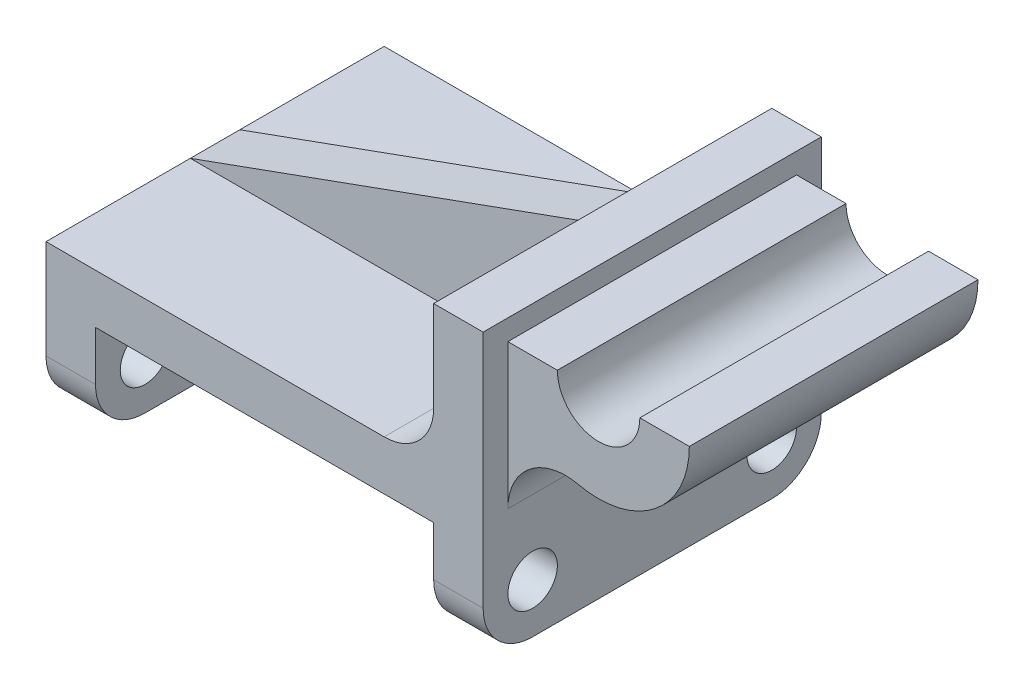
ISO-10303-21;
HEADER;
FILE_DESCRIPTION(('STEP AP214'),'2;1');
FILE_NAME('part.step','',(''),(''),'','','');
FILE_SCHEMA(('AUTOMOTIVE_DESIGN { 1 0 10303 214 1 1 1 1 }'));
ENDSEC;
DATA;
#1=APPLICATION_CONTEXT('core data for automotive mechanical design processes');
#2=APPLICATION_PROTOCOL_DEFINITION('international standard','automotive_design',2000,#1);
#3=PRODUCT_CONTEXT('',#1,'mechanical');
#4=PRODUCT('Part','Part','',(#3));
#5=PRODUCT_RELATED_PRODUCT_CATEGORY('part','',(#4));
#6=PRODUCT_DEFINITION_FORMATION('','',#4);
#7=PRODUCT_DEFINITION_CONTEXT('part definition',#1,'design');
#8=PRODUCT_DEFINITION('design','',#6,#7);
#9=PRODUCT_DEFINITION_SHAPE('','',#8);
#10=(LENGTH_UNIT() NAMED_UNIT(*) SI_UNIT(.MILLI.,.METRE.));
#11=(NAMED_UNIT(*) PLANE_ANGLE_UNIT() SI_UNIT($,.RADIAN.));
#12=(NAMED_UNIT(*) SI_UNIT($,.STERADIAN.) SOLID_ANGLE_UNIT());
#13=UNCERTAINTY_MEASURE_WITH_UNIT(LENGTH_MEASURE(1.E-05),#10,'distance_accuracy_value','');
#14=(GEOMETRIC_REPRESENTATION_CONTEXT(3) GLOBAL_UNCERTAINTY_ASSIGNED_CONTEXT((#13)) GLOBAL_UNIT_ASSIGNED_CONTEXT((#10,
#11,#12)) REPRESENTATION_CONTEXT('',''));
#15=CARTESIAN_POINT('',(0.,0.,0.));
#16=DIRECTION('',(0.,0.,1.));
#17=DIRECTION('',(1.,0.,0.));
#18=AXIS2_PLACEMENT_3D('',#15,#16,#17);
#19=CARTESIAN_POINT('',(0.,36.,0.));
#20=DIRECTION('',(0.,-1.,0.));
#21=DIRECTION('',(0.,0.,-1.));
#22=AXIS2_PLACEMENT_3D('',#19,#20,#21);
#23=PLANE('',#22);
#24=DIRECTION('',(-1.,0.,0.));
#25=VECTOR('',#24,1.);
#26=CARTESIAN_POINT('',(0.,36.,-6.));
#27=LINE('',#26,#25);
#28=CARTESIAN_POINT('',(29.,36.,-6.));
#29=VERTEX_POINT('',#28);
#30=CARTESIAN_POINT('',(-53.,36.,-6.));
#31=VERTEX_POINT('',#30);
#32=EDGE_CURVE('E217',#29,#31,#27,.T.);
#33=ORIENTED_EDGE('',*,*,#32,.F.);
#34=DIRECTION('',(0.,0.,1.));
#35=VECTOR('',#34,1.);
#36=CARTESIAN_POINT('',(29.,36.,0.));
#37=LINE('',#36,#35);
#38=CARTESIAN_POINT('',(29.,36.,-41.));
#39=VERTEX_POINT('',#38);
#40=EDGE_CURVE('E373',#29,#39,#37,.F.);
#41=ORIENTED_EDGE('',*,*,#40,.T.);
#42=DIRECTION('',(-1.,0.,0.));
#43=VECTOR('',#42,1.);
#44=CARTESIAN_POINT('',(-53.,36.,-41.));
#45=LINE('',#44,#43);
#46=CARTESIAN_POINT('',(-53.,36.,-41.));
#47=VERTEX_POINT('',#46);
#48=EDGE_CURVE('E305',#39,#47,#45,.T.);
#49=ORIENTED_EDGE('',*,*,#48,.T.);
#50=DIRECTION('',(0.,0.,1.));
#51=VECTOR('',#50,1.);
#52=CARTESIAN_POINT('',(-53.,36.,41.));
#53=LINE('',#52,#51);
#54=EDGE_CURVE('E306',#47,#31,#53,.T.);
#55=ORIENTED_EDGE('',*,*,#54,.T.);
#56=EDGE_LOOP('',(#33,#41,#49,#55));
#57=FACE_BOUND('',#56,.T.);
#58=ADVANCED_FACE('F43',(#57),#23,.F.);
#59=CARTESIAN_POINT('',(41.,36.,-41.));
#60=DIRECTION('',(-1.,0.,0.));
#61=DIRECTION('',(0.,0.,1.));
#62=AXIS2_PLACEMENT_3D('',#59,#60,#61);
#63=PLANE('',#62);
#64=DIRECTION('',(0.,-1.,0.));
#65=VECTOR('',#64,1.);
#66=CARTESIAN_POINT('',(41.,36.,-41.));
#67=LINE('',#66,#65);
#68=CARTESIAN_POINT('',(41.,70.,-41.));
#69=VERTEX_POINT('',#68);
#70=CARTESIAN_POINT('',(41.,48.,-41.));
#71=VERTEX_POINT('',#70);
#72=EDGE_CURVE('E251',#69,#71,#67,.T.);
#73=ORIENTED_EDGE('',*,*,#72,.T.);
#74=DIRECTION('',(0.,0.,1.));
#75=VECTOR('',#74,1.);
#76=CARTESIAN_POINT('',(41.,48.,-41.));
#77=LINE('',#76,#75);
#78=CARTESIAN_POINT('',(41.,48.,-6.));
#79=VERTEX_POINT('',#78);
#80=EDGE_CURVE('E216',#71,#79,#77,.T.);
#81=ORIENTED_EDGE('',*,*,#80,.T.);
#82=DIRECTION('',(0.,1.,0.));
#83=VECTOR('',#82,1.);
#84=CARTESIAN_POINT('',(41.,36.,-6.));
#85=LINE('',#84,#83);
#86=CARTESIAN_POINT('',(41.,70.,-6.));
#87=VERTEX_POINT('',#86);
#88=EDGE_CURVE('E209',#79,#87,#85,.T.);
#89=ORIENTED_EDGE('',*,*,#88,.T.);
#90=DIRECTION('',(0.,0.,1.));
#91=VECTOR('',#90,1.);
#92=CARTESIAN_POINT('',(41.,70.,-41.));
#93=LINE('',#92,#91);
#94=EDGE_CURVE('E211',#69,#87,#93,.T.);
#95=ORIENTED_EDGE('',*,*,#94,.F.);
#96=EDGE_LOOP('',(#73,#81,#89,#95));
#97=FACE_BOUND('',#96,.T.);
#98=ADVANCED_FACE('F215',(#97),#63,.T.);
#99=CARTESIAN_POINT('',(53.,65.,-35.));
#100=DIRECTION('',(0.,1.,0.));
#101=DIRECTION('',(0.,0.,1.));
#102=AXIS2_PLACEMENT_3D('',#99,#100,#101);
#103=PLANE('',#102);
#104=DIRECTION('',(-1.,0.,0.));
#105=VECTOR('',#104,1.);
#106=CARTESIAN_POINT('',(53.,65.,35.));
#107=LINE('',#106,#105);
#108=CARTESIAN_POINT('',(65.,65.,35.));
#109=VERTEX_POINT('',#108);
#110=CARTESIAN_POINT('',(53.,65.,35.));
#111=VERTEX_POINT('',#110);
#112=EDGE_CURVE('E429',#109,#111,#107,.T.);
#113=ORIENTED_EDGE('',*,*,#112,.F.);
#114=DIRECTION('',(0.,0.,1.));
#115=VECTOR('',#114,1.);
#116=CARTESIAN_POINT('',(65.,65.,-47.));
#117=LINE('',#116,#115);
#118=CARTESIAN_POINT('',(65.,65.,-35.));
#119=VERTEX_POINT('',#118);
#120=EDGE_CURVE('E401',#119,#109,#117,.T.);
#121=ORIENTED_EDGE('',*,*,#120,.F.);
#122=DIRECTION('',(-1.,0.,0.));
#123=VECTOR('',#122,1.);
#124=CARTESIAN_POINT('',(53.,65.,-35.));
#125=LINE('',#124,#123);
#126=CARTESIAN_POINT('',(53.,65.,-35.));
#127=VERTEX_POINT('',#126);
#128=EDGE_CURVE('E417',#119,#127,#125,.T.);
#129=ORIENTED_EDGE('',*,*,#128,.T.);
#130=DIRECTION('',(0.,0.,1.));
#131=VECTOR('',#130,1.);
#132=CARTESIAN_POINT('',(53.,65.,-35.));
#133=LINE('',#132,#131);
#134=EDGE_CURVE('E435',#127,#111,#133,.T.);
#135=ORIENTED_EDGE('',*,*,#134,.T.);
#136=EDGE_LOOP('',(#113,#121,#129,#135));
#137=FACE_BOUND('',#136,.T.);
#138=ADVANCED_FACE('F518',(#137),#103,.T.);
#139=CARTESIAN_POINT('',(53.,36.,41.));
#140=DIRECTION('',(-1.,0.,0.));
#141=DIRECTION('',(0.,0.,1.));
#142=AXIS2_PLACEMENT_3D('',#139,#140,#141);
#143=PLANE('',#142);
#144=DIRECTION('',(0.,0.,1.));
#145=VECTOR('',#144,1.);
#146=CARTESIAN_POINT('',(53.,29.9001424504315,-35.));
#147=LINE('',#146,#145);
#148=CARTESIAN_POINT('',(53.,29.9001424504315,-35.));
#149=VERTEX_POINT('',#148);
#150=CARTESIAN_POINT('',(53.,29.9001424504315,35.));
#151=VERTEX_POINT('',#150);
#152=EDGE_CURVE('E418',#149,#151,#147,.T.);
#153=ORIENTED_EDGE('',*,*,#152,.T.);
#154=DIRECTION('',(0.,-1.,0.));
#155=VECTOR('',#154,1.);
#156=CARTESIAN_POINT('',(53.,29.9001424504315,35.));
#157=LINE('',#156,#155);
#158=EDGE_CURVE('E403',#111,#151,#157,.T.);
#159=ORIENTED_EDGE('',*,*,#158,.F.);
#160=ORIENTED_EDGE('',*,*,#134,.F.);
#161=DIRECTION('',(0.,-1.,0.));
#162=VECTOR('',#161,1.);
#163=CARTESIAN_POINT('',(53.,29.9001424504315,-35.));
#164=LINE('',#163,#162);
#165=EDGE_CURVE('E407',#127,#149,#164,.T.);
#166=ORIENTED_EDGE('',*,*,#165,.T.);
#167=EDGE_LOOP('',(#153,#159,#160,#166));
#168=FACE_BOUND('',#167,.T.);
#169=CARTESIAN_POINT('',(53.,12.,29.));
#170=DIRECTION('',(-1.,0.,0.));
#171=DIRECTION('',(0.,0.,1.));
#172=AXIS2_PLACEMENT_3D('',#169,#170,#171);
#173=CIRCLE('',#172,6.00000000000001);
#174=CARTESIAN_POINT('',(53.,12.,35.));
#175=VERTEX_POINT('',#174);
#176=EDGE_CURVE('E258',#175,#175,#173,.T.);
#177=ORIENTED_EDGE('',*,*,#176,.T.);
#178=EDGE_LOOP('',(#177));
#179=FACE_BOUND('',#178,.T.);
#180=DIRECTION('',(0.,0.,-1.));
#181=VECTOR('',#180,1.);
#182=CARTESIAN_POINT('',(53.,0.,41.));
#183=LINE('',#182,#181);
#184=CARTESIAN_POINT('',(53.,0.,29.));
#185=VERTEX_POINT('',#184);
#186=CARTESIAN_POINT('',(53.,0.,-29.));
#187=VERTEX_POINT('',#186);
#188=EDGE_CURVE('E298',#185,#187,#183,.T.);
#189=ORIENTED_EDGE('',*,*,#188,.T.);
#190=CARTESIAN_POINT('',(53.,12.,-29.));
#191=DIRECTION('',(-1.,0.,0.));
#192=DIRECTION('',(0.,0.,1.));
#193=AXIS2_PLACEMENT_3D('',#190,#191,#192);
#194=CIRCLE('',#193,12.);
#195=CARTESIAN_POINT('',(53.,12.,-41.));
#196=VERTEX_POINT('',#195);
#197=EDGE_CURVE('E345',#187,#196,#194,.F.);
#198=ORIENTED_EDGE('',*,*,#197,.T.);
#199=DIRECTION('',(0.,-1.,0.));
#200=VECTOR('',#199,1.);
#201=CARTESIAN_POINT('',(53.,36.,-41.));
#202=LINE('',#201,#200);
#203=CARTESIAN_POINT('',(53.,70.,-41.));
#204=VERTEX_POINT('',#203);
#205=EDGE_CURVE('E322',#204,#196,#202,.T.);
#206=ORIENTED_EDGE('',*,*,#205,.F.);
#207=DIRECTION('',(0.,0.,1.));
#208=VECTOR('',#207,1.);
#209=CARTESIAN_POINT('',(53.,70.,-41.));
#210=LINE('',#209,#208);
#211=CARTESIAN_POINT('',(53.,70.,41.));
#212=VERTEX_POINT('',#211);
#213=EDGE_CURVE('E255',#204,#212,#210,.T.);
#214=ORIENTED_EDGE('',*,*,#213,.T.);
#215=DIRECTION('',(0.,-1.,0.));
#216=VECTOR('',#215,1.);
#217=CARTESIAN_POINT('',(53.,36.,41.));
#218=LINE('',#217,#216);
#219=CARTESIAN_POINT('',(53.,12.,41.));
#220=VERTEX_POINT('',#219);
#221=EDGE_CURVE('E311',#212,#220,#218,.T.);
#222=ORIENTED_EDGE('',*,*,#221,.T.);
#223=CARTESIAN_POINT('',(53.,12.,29.));
#224=DIRECTION('',(-1.,0.,0.));
#225=DIRECTION('',(0.,0.,1.));
#226=AXIS2_PLACEMENT_3D('',#223,#224,#225);
#227=CIRCLE('',#226,12.);
#228=EDGE_CURVE('E338',#220,#185,#227,.F.);
#229=ORIENTED_EDGE('',*,*,#228,.T.);
#230=EDGE_LOOP('',(#189,#198,#206,#214,#222,#229));
#231=FACE_BOUND('',#230,.T.);
#232=CARTESIAN_POINT('',(53.,12.,-29.));
#233=DIRECTION('',(-1.,0.,0.));
#234=DIRECTION('',(0.,0.,1.));
#235=AXIS2_PLACEMENT_3D('',#232,#233,#234);
#236=CIRCLE('',#235,6.);
#237=CARTESIAN_POINT('',(53.,12.,-23.));
#238=VERTEX_POINT('',#237);
#239=EDGE_CURVE('E247',#238,#238,#236,.T.);
#240=ORIENTED_EDGE('',*,*,#239,.T.);
#241=EDGE_LOOP('',(#240));
#242=FACE_BOUND('',#241,.T.);
#243=ADVANCED_FACE('F488',(#168,#179,#231,#242),#143,.F.);
#244=DIRECTION('',(1.,0.,0.));
#245=VECTOR('',#244,1.);
#246=CARTESIAN_POINT('',(-53.,36.,41.));
#247=LINE('',#246,#245);
#248=CARTESIAN_POINT('',(-53.,36.,41.));
#249=VERTEX_POINT('',#248);
#250=CARTESIAN_POINT('',(29.,36.,41.));
#251=VERTEX_POINT('',#250);
#252=EDGE_CURVE('E307',#249,#251,#247,.T.);
#253=ORIENTED_EDGE('',*,*,#252,.T.);
#254=DIRECTION('',(0.,0.,1.));
#255=VECTOR('',#254,1.);
#256=CARTESIAN_POINT('',(29.,36.,0.));
#257=LINE('',#256,#255);
#258=CARTESIAN_POINT('',(29.,36.,6.));
#259=VERTEX_POINT('',#258);
#260=EDGE_CURVE('E64',#251,#259,#257,.F.);
#261=ORIENTED_EDGE('',*,*,#260,.T.);
#262=DIRECTION('',(-1.,0.,0.));
#263=VECTOR('',#262,1.);
#264=CARTESIAN_POINT('',(0.,36.,6.));
#265=LINE('',#264,#263);
#266=CARTESIAN_POINT('',(-53.,36.,6.));
#267=VERTEX_POINT('',#266);
#268=EDGE_CURVE('E391',#259,#267,#265,.T.);
#269=ORIENTED_EDGE('',*,*,#268,.T.);
#270=EDGE_CURVE('E302',#267,#249,#53,.T.);
#271=ORIENTED_EDGE('',*,*,#270,.T.);
#272=EDGE_LOOP('',(#253,#261,#269,#271));
#273=FACE_BOUND('',#272,.T.);
#274=ADVANCED_FACE('F451',(#273),#23,.F.);
#275=CARTESIAN_POINT('',(0.,0.,0.));
#276=DIRECTION('',(0.,-1.,0.));
#277=DIRECTION('',(0.,0.,-1.));
#278=AXIS2_PLACEMENT_3D('',#275,#276,#277);
#279=PLANE('',#278);
#280=DIRECTION('',(1.,0.,0.));
#281=VECTOR('',#280,1.);
#282=CARTESIAN_POINT('',(-53.,0.,29.));
#283=LINE('',#282,#281);
#284=CARTESIAN_POINT('',(-41.,0.,29.));
#285=VERTEX_POINT('',#284);
#286=CARTESIAN_POINT('',(-53.,0.,29.));
#287=VERTEX_POINT('',#286);
#288=EDGE_CURVE('E351',#285,#287,#283,.F.);
#289=ORIENTED_EDGE('',*,*,#288,.T.);
#290=DIRECTION('',(0.,0.,1.));
#291=VECTOR('',#290,1.);
#292=CARTESIAN_POINT('',(-53.,0.,41.));
#293=LINE('',#292,#291);
#294=CARTESIAN_POINT('',(-53.,0.,-29.));
#295=VERTEX_POINT('',#294);
#296=EDGE_CURVE('E304',#295,#287,#293,.T.);
#297=ORIENTED_EDGE('',*,*,#296,.F.);
#298=DIRECTION('',(-1.,0.,0.));
#299=VECTOR('',#298,1.);
#300=CARTESIAN_POINT('',(-41.,0.,-29.));
#301=LINE('',#300,#299);
#302=CARTESIAN_POINT('',(-41.,0.,-29.));
#303=VERTEX_POINT('',#302);
#304=EDGE_CURVE('E357',#295,#303,#301,.F.);
#305=ORIENTED_EDGE('',*,*,#304,.T.);
#306=DIRECTION('',(0.,0.,1.));
#307=VECTOR('',#306,1.);
#308=CARTESIAN_POINT('',(-41.,0.,-41.));
#309=LINE('',#308,#307);
#310=EDGE_CURVE('E287',#303,#285,#309,.T.);
#311=ORIENTED_EDGE('',*,*,#310,.T.);
#312=EDGE_LOOP('',(#289,#297,#305,#311));
#313=FACE_BOUND('',#312,.T.);
#314=ADVANCED_FACE('F505',(#313),#279,.T.);
#315=CARTESIAN_POINT('',(-53.,36.,-41.));
#316=DIRECTION('',(0.,0.,1.));
#317=DIRECTION('',(1.,0.,0.));
#318=AXIS2_PLACEMENT_3D('',#315,#316,#317);
#319=PLANE('',#318);
#320=ORIENTED_EDGE('',*,*,#205,.T.);
#321=DIRECTION('',(-1.,0.,0.));
#322=VECTOR('',#321,1.);
#323=CARTESIAN_POINT('',(41.,12.,-41.));
#324=LINE('',#323,#322);
#325=CARTESIAN_POINT('',(41.,12.,-41.));
#326=VERTEX_POINT('',#325);
#327=EDGE_CURVE('E326',#196,#326,#324,.T.);
#328=ORIENTED_EDGE('',*,*,#327,.T.);
#329=DIRECTION('',(0.,1.,0.));
#330=VECTOR('',#329,1.);
#331=CARTESIAN_POINT('',(41.,0.,-41.));
#332=LINE('',#331,#330);
#333=CARTESIAN_POINT('',(41.,24.,-41.));
#334=VERTEX_POINT('',#333);
#335=EDGE_CURVE('E278',#326,#334,#332,.T.);
#336=ORIENTED_EDGE('',*,*,#335,.T.);
#337=DIRECTION('',(-1.,0.,0.));
#338=VECTOR('',#337,1.);
#339=CARTESIAN_POINT('',(-41.,24.,-41.));
#340=LINE('',#339,#338);
#341=CARTESIAN_POINT('',(-41.,24.,-41.));
#342=VERTEX_POINT('',#341);
#343=EDGE_CURVE('E285',#334,#342,#340,.T.);
#344=ORIENTED_EDGE('',*,*,#343,.T.);
#345=DIRECTION('',(0.,-1.,0.));
#346=VECTOR('',#345,1.);
#347=CARTESIAN_POINT('',(-41.,0.,-41.));
#348=LINE('',#347,#346);
#349=CARTESIAN_POINT('',(-41.,12.,-41.));
#350=VERTEX_POINT('',#349);
#351=EDGE_CURVE('E280',#342,#350,#348,.T.);
#352=ORIENTED_EDGE('',*,*,#351,.T.);
#353=DIRECTION('',(-1.,0.,0.));
#354=VECTOR('',#353,1.);
#355=CARTESIAN_POINT('',(-53.,12.,-41.));
#356=LINE('',#355,#354);
#357=CARTESIAN_POINT('',(-53.,12.,-41.));
#358=VERTEX_POINT('',#357);
#359=EDGE_CURVE('E321',#350,#358,#356,.T.);
#360=ORIENTED_EDGE('',*,*,#359,.T.);
#361=DIRECTION('',(0.,-1.,0.));
#362=VECTOR('',#361,1.);
#363=CARTESIAN_POINT('',(-53.,36.,-41.));
#364=LINE('',#363,#362);
#365=EDGE_CURVE('E319',#47,#358,#364,.T.);
#366=ORIENTED_EDGE('',*,*,#365,.F.);
#367=ORIENTED_EDGE('',*,*,#48,.F.);
#368=CARTESIAN_POINT('',(29.,48.,-41.));
#369=DIRECTION('',(0.,0.,1.));
#370=DIRECTION('',(1.,0.,0.));
#371=AXIS2_PLACEMENT_3D('',#368,#369,#370);
#372=CIRCLE('',#371,12.);
#373=EDGE_CURVE('E51',#39,#71,#372,.T.);
#374=ORIENTED_EDGE('',*,*,#373,.T.);
#375=ORIENTED_EDGE('',*,*,#72,.F.);
#376=DIRECTION('',(-1.,0.,0.));
#377=VECTOR('',#376,1.);
#378=CARTESIAN_POINT('',(53.,70.,-41.));
#379=LINE('',#378,#377);
#380=EDGE_CURVE('E244',#204,#69,#379,.T.);
#381=ORIENTED_EDGE('',*,*,#380,.F.);
#382=EDGE_LOOP('',(#320,#328,#336,#344,#352,#360,#366,#367,#374,#375,#381));
#383=FACE_BOUND('',#382,.T.);
#384=ADVANCED_FACE('F384',(#383),#319,.F.);
#385=CARTESIAN_POINT('',(-53.,36.,41.));
#386=DIRECTION('',(1.,0.,0.));
#387=DIRECTION('',(0.,0.,-1.));
#388=AXIS2_PLACEMENT_3D('',#385,#386,#387);
#389=PLANE('',#388);
#390=CARTESIAN_POINT('',(-53.,12.,29.));
#391=DIRECTION('',(-1.,0.,0.));
#392=DIRECTION('',(0.,0.,1.));
#393=AXIS2_PLACEMENT_3D('',#390,#391,#392);
#394=CIRCLE('',#393,6.00000000000001);
#395=CARTESIAN_POINT('',(-53.,12.,35.));
#396=VERTEX_POINT('',#395);
#397=EDGE_CURVE('E263',#396,#396,#394,.T.);
#398=ORIENTED_EDGE('',*,*,#397,.F.);
#399=EDGE_LOOP('',(#398));
#400=FACE_BOUND('',#399,.T.);
#401=ORIENTED_EDGE('',*,*,#270,.F.);
#402=DIRECTION('',(0.,0.,1.));
#403=VECTOR('',#402,1.);
#404=CARTESIAN_POINT('',(-53.,36.,41.));
#405=LINE('',#404,#403);
#406=EDGE_CURVE('E397',#31,#267,#405,.T.);
#407=ORIENTED_EDGE('',*,*,#406,.F.);
#408=ORIENTED_EDGE('',*,*,#54,.F.);
#409=ORIENTED_EDGE('',*,*,#365,.T.);
#410=CARTESIAN_POINT('',(-53.,12.,-29.));
#411=DIRECTION('',(1.,0.,0.));
#412=DIRECTION('',(0.,0.,-1.));
#413=AXIS2_PLACEMENT_3D('',#410,#411,#412);
#414=CIRCLE('',#413,12.);
#415=EDGE_CURVE('E355',#358,#295,#414,.F.);
#416=ORIENTED_EDGE('',*,*,#415,.T.);
#417=ORIENTED_EDGE('',*,*,#296,.T.);
#418=CARTESIAN_POINT('',(-53.,12.,29.));
#419=DIRECTION('',(1.,0.,0.));
#420=DIRECTION('',(0.,0.,-1.));
#421=AXIS2_PLACEMENT_3D('',#418,#419,#420);
#422=CIRCLE('',#421,12.);
#423=CARTESIAN_POINT('',(-53.,12.,41.));
#424=VERTEX_POINT('',#423);
#425=EDGE_CURVE('E347',#287,#424,#422,.F.);
#426=ORIENTED_EDGE('',*,*,#425,.T.);
#427=DIRECTION('',(0.,-1.,0.));
#428=VECTOR('',#427,1.);
#429=CARTESIAN_POINT('',(-53.,36.,41.));
#430=LINE('',#429,#428);
#431=EDGE_CURVE('E314',#249,#424,#430,.T.);
#432=ORIENTED_EDGE('',*,*,#431,.F.);
#433=EDGE_LOOP('',(#401,#407,#408,#409,#416,#417,#426,#432));
#434=FACE_BOUND('',#433,.T.);
#435=CARTESIAN_POINT('',(-53.,12.,-29.));
#436=DIRECTION('',(-1.,0.,0.));
#437=DIRECTION('',(0.,0.,1.));
#438=AXIS2_PLACEMENT_3D('',#435,#436,#437);
#439=CIRCLE('',#438,6.);
#440=CARTESIAN_POINT('',(-53.,12.,-23.));
#441=VERTEX_POINT('',#440);
#442=EDGE_CURVE('E246',#441,#441,#439,.T.);
#443=ORIENTED_EDGE('',*,*,#442,.F.);
#444=EDGE_LOOP('',(#443));
#445=FACE_BOUND('',#444,.T.);
#446=ADVANCED_FACE('F456',(#400,#434,#445),#389,.F.);
#447=CARTESIAN_POINT('',(-53.,36.,41.));
#448=DIRECTION('',(0.,0.,-1.));
#449=DIRECTION('',(-1.,0.,0.));
#450=AXIS2_PLACEMENT_3D('',#447,#448,#449);
#451=PLANE('',#450);
#452=DIRECTION('',(0.,1.,0.));
#453=VECTOR('',#452,1.);
#454=CARTESIAN_POINT('',(41.,0.,41.));
#455=LINE('',#454,#453);
#456=CARTESIAN_POINT('',(41.,12.,41.));
#457=VERTEX_POINT('',#456);
#458=CARTESIAN_POINT('',(41.,24.,41.));
#459=VERTEX_POINT('',#458);
#460=EDGE_CURVE('E286',#457,#459,#455,.T.);
#461=ORIENTED_EDGE('',*,*,#460,.F.);
#462=DIRECTION('',(1.,0.,0.));
#463=VECTOR('',#462,1.);
#464=CARTESIAN_POINT('',(53.,12.,41.));
#465=LINE('',#464,#463);
#466=EDGE_CURVE('E346',#457,#220,#465,.T.);
#467=ORIENTED_EDGE('',*,*,#466,.T.);
#468=ORIENTED_EDGE('',*,*,#221,.F.);
#469=DIRECTION('',(-1.,0.,0.));
#470=VECTOR('',#469,1.);
#471=CARTESIAN_POINT('',(53.,70.,41.));
#472=LINE('',#471,#470);
#473=CARTESIAN_POINT('',(41.,70.,41.));
#474=VERTEX_POINT('',#473);
#475=EDGE_CURVE('E432',#212,#474,#472,.T.);
#476=ORIENTED_EDGE('',*,*,#475,.T.);
#477=DIRECTION('',(0.,-1.,0.));
#478=VECTOR('',#477,1.);
#479=CARTESIAN_POINT('',(41.,36.,41.));
#480=LINE('',#479,#478);
#481=CARTESIAN_POINT('',(41.,48.,41.));
#482=VERTEX_POINT('',#481);
#483=EDGE_CURVE('E439',#474,#482,#480,.T.);
#484=ORIENTED_EDGE('',*,*,#483,.T.);
#485=CARTESIAN_POINT('',(29.,48.,41.));
#486=DIRECTION('',(0.,0.,-1.));
#487=DIRECTION('',(-1.,0.,0.));
#488=AXIS2_PLACEMENT_3D('',#485,#486,#487);
#489=CIRCLE('',#488,12.);
#490=EDGE_CURVE('E11',#482,#251,#489,.T.);
#491=ORIENTED_EDGE('',*,*,#490,.T.);
#492=ORIENTED_EDGE('',*,*,#252,.F.);
#493=ORIENTED_EDGE('',*,*,#431,.T.);
#494=DIRECTION('',(1.,0.,0.));
#495=VECTOR('',#494,1.);
#496=CARTESIAN_POINT('',(-41.,12.,41.));
#497=LINE('',#496,#495);
#498=CARTESIAN_POINT('',(-41.,12.,41.));
#499=VERTEX_POINT('',#498);
#500=EDGE_CURVE('E341',#424,#499,#497,.T.);
#501=ORIENTED_EDGE('',*,*,#500,.T.);
#502=DIRECTION('',(0.,-1.,0.));
#503=VECTOR('',#502,1.);
#504=CARTESIAN_POINT('',(-41.,0.,41.));
#505=LINE('',#504,#503);
#506=CARTESIAN_POINT('',(-41.,24.,41.));
#507=VERTEX_POINT('',#506);
#508=EDGE_CURVE('E277',#507,#499,#505,.T.);
#509=ORIENTED_EDGE('',*,*,#508,.F.);
#510=DIRECTION('',(-1.,0.,0.));
#511=VECTOR('',#510,1.);
#512=CARTESIAN_POINT('',(-41.,24.,41.));
#513=LINE('',#512,#511);
#514=EDGE_CURVE('E284',#459,#507,#513,.T.);
#515=ORIENTED_EDGE('',*,*,#514,.F.);
#516=EDGE_LOOP('',(#461,#467,#468,#476,#484,#491,#492,#493,#501,#509,#515));
#517=FACE_BOUND('',#516,.T.);
#518=ADVANCED_FACE('F443',(#517),#451,.F.);
#519=DIRECTION('',(1.,0.,0.));
#520=VECTOR('',#519,1.);
#521=CARTESIAN_POINT('',(41.,0.,29.));
#522=LINE('',#521,#520);
#523=CARTESIAN_POINT('',(41.,0.,29.));
#524=VERTEX_POINT('',#523);
#525=EDGE_CURVE('E331',#185,#524,#522,.F.);
#526=ORIENTED_EDGE('',*,*,#525,.T.);
#527=DIRECTION('',(0.,0.,1.));
#528=VECTOR('',#527,1.);
#529=CARTESIAN_POINT('',(41.,0.,-41.));
#530=LINE('',#529,#528);
#531=CARTESIAN_POINT('',(41.,0.,-29.));
#532=VERTEX_POINT('',#531);
#533=EDGE_CURVE('E299',#532,#524,#530,.T.);
#534=ORIENTED_EDGE('',*,*,#533,.F.);
#535=DIRECTION('',(-1.,0.,0.));
#536=VECTOR('',#535,1.);
#537=CARTESIAN_POINT('',(53.,0.,-29.));
#538=LINE('',#537,#536);
#539=EDGE_CURVE('E340',#532,#187,#538,.F.);
#540=ORIENTED_EDGE('',*,*,#539,.T.);
#541=ORIENTED_EDGE('',*,*,#188,.F.);
#542=EDGE_LOOP('',(#526,#534,#540,#541));
#543=FACE_BOUND('',#542,.T.);
#544=ADVANCED_FACE('F489',(#543),#279,.T.);
#545=CARTESIAN_POINT('',(-41.,0.,-41.));
#546=DIRECTION('',(-1.,0.,0.));
#547=DIRECTION('',(0.,0.,1.));
#548=AXIS2_PLACEMENT_3D('',#545,#546,#547);
#549=PLANE('',#548);
#550=CARTESIAN_POINT('',(-41.,12.,29.));
#551=DIRECTION('',(-1.,0.,0.));
#552=DIRECTION('',(0.,0.,1.));
#553=AXIS2_PLACEMENT_3D('',#550,#551,#552);
#554=CIRCLE('',#553,6.00000000000001);
#555=CARTESIAN_POINT('',(-41.,12.,35.));
#556=VERTEX_POINT('',#555);
#557=EDGE_CURVE('E271',#556,#556,#554,.T.);
#558=ORIENTED_EDGE('',*,*,#557,.T.);
#559=EDGE_LOOP('',(#558));
#560=FACE_BOUND('',#559,.T.);
#561=CARTESIAN_POINT('',(-41.,12.,29.));
#562=DIRECTION('',(-1.,0.,0.));
#563=DIRECTION('',(0.,0.,1.));
#564=AXIS2_PLACEMENT_3D('',#561,#562,#563);
#565=CIRCLE('',#564,12.);
#566=EDGE_CURVE('E360',#499,#285,#565,.F.);
#567=ORIENTED_EDGE('',*,*,#566,.T.);
#568=ORIENTED_EDGE('',*,*,#310,.F.);
#569=CARTESIAN_POINT('',(-41.,12.,-29.));
#570=DIRECTION('',(-1.,0.,0.));
#571=DIRECTION('',(0.,0.,1.));
#572=AXIS2_PLACEMENT_3D('',#569,#570,#571);
#573=CIRCLE('',#572,12.);
#574=EDGE_CURVE('E365',#303,#350,#573,.F.);
#575=ORIENTED_EDGE('',*,*,#574,.T.);
#576=ORIENTED_EDGE('',*,*,#351,.F.);
#577=DIRECTION('',(0.,0.,1.));
#578=VECTOR('',#577,1.);
#579=CARTESIAN_POINT('',(-41.,24.,-41.));
#580=LINE('',#579,#578);
#581=EDGE_CURVE('E295',#342,#507,#580,.T.);
#582=ORIENTED_EDGE('',*,*,#581,.T.);
#583=ORIENTED_EDGE('',*,*,#508,.T.);
#584=EDGE_LOOP('',(#567,#568,#575,#576,#582,#583));
#585=FACE_BOUND('',#584,.T.);
#586=CARTESIAN_POINT('',(-41.,12.,-29.));
#587=DIRECTION('',(-1.,0.,0.));
#588=DIRECTION('',(0.,0.,1.));
#589=AXIS2_PLACEMENT_3D('',#586,#587,#588);
#590=CIRCLE('',#589,6.);
#591=CARTESIAN_POINT('',(-41.,12.,-23.));
#592=VERTEX_POINT('',#591);
#593=EDGE_CURVE('E266',#592,#592,#590,.T.);
#594=ORIENTED_EDGE('',*,*,#593,.T.);
#595=EDGE_LOOP('',(#594));
#596=FACE_BOUND('',#595,.T.);
#597=ADVANCED_FACE('F470',(#560,#585,#596),#549,.F.);
#598=CARTESIAN_POINT('',(-41.,24.,-41.));
#599=DIRECTION('',(0.,1.,0.));
#600=DIRECTION('',(0.,0.,1.));
#601=AXIS2_PLACEMENT_3D('',#598,#599,#600);
#602=PLANE('',#601);
#603=ORIENTED_EDGE('',*,*,#514,.T.);
#604=ORIENTED_EDGE('',*,*,#581,.F.);
#605=ORIENTED_EDGE('',*,*,#343,.F.);
#606=DIRECTION('',(0.,0.,1.));
#607=VECTOR('',#606,1.);
#608=CARTESIAN_POINT('',(41.,24.,-41.));
#609=LINE('',#608,#607);
#610=EDGE_CURVE('E300',#334,#459,#609,.T.);
#611=ORIENTED_EDGE('',*,*,#610,.T.);
#612=EDGE_LOOP('',(#603,#604,#605,#611));
#613=FACE_BOUND('',#612,.T.);
#614=ADVANCED_FACE('F471',(#613),#602,.F.);
#615=CARTESIAN_POINT('',(41.,0.,-41.));
#616=DIRECTION('',(1.,0.,0.));
#617=DIRECTION('',(0.,0.,-1.));
#618=AXIS2_PLACEMENT_3D('',#615,#616,#617);
#619=PLANE('',#618);
#620=CARTESIAN_POINT('',(41.,12.,29.));
#621=DIRECTION('',(1.,0.,0.));
#622=DIRECTION('',(0.,0.,-1.));
#623=AXIS2_PLACEMENT_3D('',#620,#621,#622);
#624=CIRCLE('',#623,6.00000000000001);
#625=CARTESIAN_POINT('',(41.,12.,23.));
#626=VERTEX_POINT('',#625);
#627=EDGE_CURVE('E275',#626,#626,#624,.T.);
#628=ORIENTED_EDGE('',*,*,#627,.T.);
#629=EDGE_LOOP('',(#628));
#630=FACE_BOUND('',#629,.T.);
#631=ORIENTED_EDGE('',*,*,#460,.T.);
#632=ORIENTED_EDGE('',*,*,#610,.F.);
#633=ORIENTED_EDGE('',*,*,#335,.F.);
#634=CARTESIAN_POINT('',(41.,12.,-29.));
#635=DIRECTION('',(1.,0.,0.));
#636=DIRECTION('',(0.,0.,-1.));
#637=AXIS2_PLACEMENT_3D('',#634,#635,#636);
#638=CIRCLE('',#637,12.);
#639=EDGE_CURVE('E335',#326,#532,#638,.F.);
#640=ORIENTED_EDGE('',*,*,#639,.T.);
#641=ORIENTED_EDGE('',*,*,#533,.T.);
#642=CARTESIAN_POINT('',(41.,12.,29.));
#643=DIRECTION('',(1.,0.,0.));
#644=DIRECTION('',(0.,0.,-1.));
#645=AXIS2_PLACEMENT_3D('',#642,#643,#644);
#646=CIRCLE('',#645,12.);
#647=EDGE_CURVE('E327',#524,#457,#646,.F.);
#648=ORIENTED_EDGE('',*,*,#647,.T.);
#649=EDGE_LOOP('',(#631,#632,#633,#640,#641,#648));
#650=FACE_BOUND('',#649,.T.);
#651=CARTESIAN_POINT('',(41.,12.,-29.));
#652=DIRECTION('',(1.,0.,0.));
#653=DIRECTION('',(0.,0.,-1.));
#654=AXIS2_PLACEMENT_3D('',#651,#652,#653);
#655=CIRCLE('',#654,6.);
#656=CARTESIAN_POINT('',(41.,12.,-35.));
#657=VERTEX_POINT('',#656);
#658=EDGE_CURVE('E265',#657,#657,#655,.T.);
#659=ORIENTED_EDGE('',*,*,#658,.T.);
#660=EDGE_LOOP('',(#659));
#661=FACE_BOUND('',#660,.T.);
#662=ADVANCED_FACE('F478',(#630,#650,#661),#619,.F.);
#663=CARTESIAN_POINT('',(-53.,12.,-29.));
#664=DIRECTION('',(1.,0.,0.));
#665=DIRECTION('',(0.,0.,-1.));
#666=AXIS2_PLACEMENT_3D('',#663,#664,#665);
#667=CYLINDRICAL_SURFACE('',#666,12.);
#668=ORIENTED_EDGE('',*,*,#197,.F.);
#669=ORIENTED_EDGE('',*,*,#539,.F.);
#670=ORIENTED_EDGE('',*,*,#639,.F.);
#671=ORIENTED_EDGE('',*,*,#327,.F.);
#672=EDGE_LOOP('',(#668,#669,#670,#671));
#673=FACE_BOUND('',#672,.T.);
#674=ADVANCED_FACE('F492',(#673),#667,.T.);
#675=CARTESIAN_POINT('',(-53.,12.,29.));
#676=DIRECTION('',(-1.,0.,0.));
#677=DIRECTION('',(0.,0.,1.));
#678=AXIS2_PLACEMENT_3D('',#675,#676,#677);
#679=CYLINDRICAL_SURFACE('',#678,12.);
#680=ORIENTED_EDGE('',*,*,#647,.F.);
#681=ORIENTED_EDGE('',*,*,#525,.F.);
#682=ORIENTED_EDGE('',*,*,#228,.F.);
#683=ORIENTED_EDGE('',*,*,#466,.F.);
#684=EDGE_LOOP('',(#680,#681,#682,#683));
#685=FACE_BOUND('',#684,.T.);
#686=ADVANCED_FACE('F483',(#685),#679,.T.);
#687=CARTESIAN_POINT('',(-53.,12.,-29.));
#688=DIRECTION('',(1.,0.,0.));
#689=DIRECTION('',(0.,0.,-1.));
#690=AXIS2_PLACEMENT_3D('',#687,#688,#689);
#691=CYLINDRICAL_SURFACE('',#690,12.);
#692=ORIENTED_EDGE('',*,*,#574,.F.);
#693=ORIENTED_EDGE('',*,*,#304,.F.);
#694=ORIENTED_EDGE('',*,*,#415,.F.);
#695=ORIENTED_EDGE('',*,*,#359,.F.);
#696=EDGE_LOOP('',(#692,#693,#694,#695));
#697=FACE_BOUND('',#696,.T.);
#698=ADVANCED_FACE('F498',(#697),#691,.T.);
#699=CARTESIAN_POINT('',(-53.,12.,29.));
#700=DIRECTION('',(-1.,0.,0.));
#701=DIRECTION('',(0.,0.,1.));
#702=AXIS2_PLACEMENT_3D('',#699,#700,#701);
#703=CYLINDRICAL_SURFACE('',#702,12.);
#704=ORIENTED_EDGE('',*,*,#425,.F.);
#705=ORIENTED_EDGE('',*,*,#288,.F.);
#706=ORIENTED_EDGE('',*,*,#566,.F.);
#707=ORIENTED_EDGE('',*,*,#500,.F.);
#708=EDGE_LOOP('',(#704,#705,#706,#707));
#709=FACE_BOUND('',#708,.T.);
#710=ADVANCED_FACE('F464',(#709),#703,.T.);
#711=CARTESIAN_POINT('',(53.,12.,-29.));
#712=DIRECTION('',(-1.,0.,0.));
#713=DIRECTION('',(0.,0.,1.));
#714=AXIS2_PLACEMENT_3D('',#711,#712,#713);
#715=CYLINDRICAL_SURFACE('',#714,6.);
#716=ORIENTED_EDGE('',*,*,#239,.F.);
#717=EDGE_LOOP('',(#716));
#718=FACE_BOUND('',#717,.T.);
#719=ORIENTED_EDGE('',*,*,#658,.F.);
#720=EDGE_LOOP('',(#719));
#721=FACE_BOUND('',#720,.T.);
#722=ADVANCED_FACE('F540',(#718,#721),#715,.F.);
#723=CARTESIAN_POINT('',(53.,12.,29.));
#724=DIRECTION('',(-1.,0.,0.));
#725=DIRECTION('',(0.,0.,1.));
#726=AXIS2_PLACEMENT_3D('',#723,#724,#725);
#727=CYLINDRICAL_SURFACE('',#726,6.00000000000001);
#728=ORIENTED_EDGE('',*,*,#176,.F.);
#729=EDGE_LOOP('',(#728));
#730=FACE_BOUND('',#729,.T.);
#731=ORIENTED_EDGE('',*,*,#627,.F.);
#732=EDGE_LOOP('',(#731));
#733=FACE_BOUND('',#732,.T.);
#734=ADVANCED_FACE('F533',(#730,#733),#727,.F.);
#735=ORIENTED_EDGE('',*,*,#442,.T.);
#736=EDGE_LOOP('',(#735));
#737=FACE_BOUND('',#736,.T.);
#738=ORIENTED_EDGE('',*,*,#593,.F.);
#739=EDGE_LOOP('',(#738));
#740=FACE_BOUND('',#739,.T.);
#741=ADVANCED_FACE('F532',(#737,#740),#715,.F.);
#742=ORIENTED_EDGE('',*,*,#397,.T.);
#743=EDGE_LOOP('',(#742));
#744=FACE_BOUND('',#743,.T.);
#745=ORIENTED_EDGE('',*,*,#557,.F.);
#746=EDGE_LOOP('',(#745));
#747=FACE_BOUND('',#746,.T.);
#748=ADVANCED_FACE('F534',(#744,#747),#727,.F.);
#749=DIRECTION('',(0.,1.,0.));
#750=VECTOR('',#749,1.);
#751=CARTESIAN_POINT('',(41.,36.,6.));
#752=LINE('',#751,#750);
#753=CARTESIAN_POINT('',(41.,48.,6.));
#754=VERTEX_POINT('',#753);
#755=CARTESIAN_POINT('',(41.,70.,6.));
#756=VERTEX_POINT('',#755);
#757=EDGE_CURVE('E388',#754,#756,#752,.T.);
#758=ORIENTED_EDGE('',*,*,#757,.F.);
#759=DIRECTION('',(0.,0.,1.));
#760=VECTOR('',#759,1.);
#761=CARTESIAN_POINT('',(41.,48.,-41.));
#762=LINE('',#761,#760);
#763=EDGE_CURVE('E374',#754,#482,#762,.T.);
#764=ORIENTED_EDGE('',*,*,#763,.T.);
#765=ORIENTED_EDGE('',*,*,#483,.F.);
#766=EDGE_CURVE('E232',#756,#474,#93,.T.);
#767=ORIENTED_EDGE('',*,*,#766,.F.);
#768=EDGE_LOOP('',(#758,#764,#765,#767));
#769=FACE_BOUND('',#768,.T.);
#770=ADVANCED_FACE('F450',(#769),#63,.T.);
#771=CARTESIAN_POINT('',(53.,70.,-41.));
#772=DIRECTION('',(0.,1.,0.));
#773=DIRECTION('',(0.,0.,1.));
#774=AXIS2_PLACEMENT_3D('',#771,#772,#773);
#775=PLANE('',#774);
#776=ORIENTED_EDGE('',*,*,#475,.F.);
#777=ORIENTED_EDGE('',*,*,#213,.F.);
#778=ORIENTED_EDGE('',*,*,#380,.T.);
#779=ORIENTED_EDGE('',*,*,#94,.T.);
#780=EDGE_CURVE('E227',#87,#756,#93,.T.);
#781=ORIENTED_EDGE('',*,*,#780,.T.);
#782=ORIENTED_EDGE('',*,*,#766,.T.);
#783=EDGE_LOOP('',(#776,#777,#778,#779,#781,#782));
#784=FACE_BOUND('',#783,.T.);
#785=ADVANCED_FACE('F245',(#784),#775,.T.);
#786=CARTESIAN_POINT('',(97.,65.,35.));
#787=VERTEX_POINT('',#786);
#788=CARTESIAN_POINT('',(85.,65.,35.));
#789=VERTEX_POINT('',#788);
#790=EDGE_CURVE('E408',#787,#789,#107,.T.);
#791=ORIENTED_EDGE('',*,*,#790,.F.);
#792=DIRECTION('',(0.,0.,1.));
#793=VECTOR('',#792,1.);
#794=CARTESIAN_POINT('',(97.,65.,-35.));
#795=LINE('',#794,#793);
#796=CARTESIAN_POINT('',(97.,65.,-35.));
#797=VERTEX_POINT('',#796);
#798=EDGE_CURVE('E434',#797,#787,#795,.T.);
#799=ORIENTED_EDGE('',*,*,#798,.F.);
#800=CARTESIAN_POINT('',(85.,65.,-35.));
#801=VERTEX_POINT('',#800);
#802=EDGE_CURVE('E420',#797,#801,#125,.T.);
#803=ORIENTED_EDGE('',*,*,#802,.T.);
#804=DIRECTION('',(0.,0.,1.));
#805=VECTOR('',#804,1.);
#806=CARTESIAN_POINT('',(85.,65.,-47.));
#807=LINE('',#806,#805);
#808=EDGE_CURVE('E402',#789,#801,#807,.F.);
#809=ORIENTED_EDGE('',*,*,#808,.F.);
#810=EDGE_LOOP('',(#791,#799,#803,#809));
#811=FACE_BOUND('',#810,.T.);
#812=ADVANCED_FACE('F541',(#811),#103,.T.);
#813=CARTESIAN_POINT('',(75.,65.,-35.));
#814=DIRECTION('',(0.,0.,1.));
#815=DIRECTION('',(1.,0.,0.));
#816=AXIS2_PLACEMENT_3D('',#813,#814,#815);
#817=CYLINDRICAL_SURFACE('',#816,22.);
#818=CARTESIAN_POINT('',(75.,65.,35.));
#819=DIRECTION('',(0.,0.,1.));
#820=DIRECTION('',(1.,0.,0.));
#821=AXIS2_PLACEMENT_3D('',#818,#819,#820);
#822=CIRCLE('',#821,22.);
#823=CARTESIAN_POINT('',(70.1111111111111,43.5500870530415,35.));
#824=VERTEX_POINT('',#823);
#825=EDGE_CURVE('E428',#824,#787,#822,.T.);
#826=ORIENTED_EDGE('',*,*,#825,.F.);
#827=DIRECTION('',(0.,0.,1.));
#828=VECTOR('',#827,1.);
#829=CARTESIAN_POINT('',(70.1111111111111,43.5500870530415,-35.));
#830=LINE('',#829,#828);
#831=CARTESIAN_POINT('',(70.1111111111111,43.5500870530415,-35.));
#832=VERTEX_POINT('',#831);
#833=EDGE_CURVE('E440',#832,#824,#830,.T.);
#834=ORIENTED_EDGE('',*,*,#833,.F.);
#835=CARTESIAN_POINT('',(75.,65.,-35.));
#836=DIRECTION('',(0.,0.,1.));
#837=DIRECTION('',(1.,0.,0.));
#838=AXIS2_PLACEMENT_3D('',#835,#836,#837);
#839=CIRCLE('',#838,22.);
#840=EDGE_CURVE('E415',#832,#797,#839,.T.);
#841=ORIENTED_EDGE('',*,*,#840,.T.);
#842=ORIENTED_EDGE('',*,*,#798,.T.);
#843=EDGE_LOOP('',(#826,#834,#841,#842));
#844=FACE_BOUND('',#843,.T.);
#845=ADVANCED_FACE('F546',(#844),#817,.T.);
#846=CARTESIAN_POINT('',(67.,29.9001424504315,-35.));
#847=DIRECTION('',(0.,0.,1.));
#848=DIRECTION('',(1.,0.,0.));
#849=AXIS2_PLACEMENT_3D('',#846,#847,#848);
#850=CYLINDRICAL_SURFACE('',#849,14.);
#851=CARTESIAN_POINT('',(67.,29.9001424504315,35.));
#852=DIRECTION('',(0.,0.,-1.));
#853=DIRECTION('',(1.,0.,0.));
#854=AXIS2_PLACEMENT_3D('',#851,#852,#853);
#855=CIRCLE('',#854,14.);
#856=EDGE_CURVE('E421',#151,#824,#855,.T.);
#857=ORIENTED_EDGE('',*,*,#856,.F.);
#858=ORIENTED_EDGE('',*,*,#152,.F.);
#859=CARTESIAN_POINT('',(67.,29.9001424504315,-35.));
#860=DIRECTION('',(0.,0.,-1.));
#861=DIRECTION('',(1.,0.,0.));
#862=AXIS2_PLACEMENT_3D('',#859,#860,#861);
#863=CIRCLE('',#862,14.);
#864=EDGE_CURVE('E406',#149,#832,#863,.T.);
#865=ORIENTED_EDGE('',*,*,#864,.T.);
#866=ORIENTED_EDGE('',*,*,#833,.T.);
#867=EDGE_LOOP('',(#857,#858,#865,#866));
#868=FACE_BOUND('',#867,.T.);
#869=ADVANCED_FACE('F542',(#868),#850,.F.);
#870=CARTESIAN_POINT('',(75.,65.,-35.));
#871=DIRECTION('',(0.,0.,1.));
#872=DIRECTION('',(1.,0.,0.));
#873=AXIS2_PLACEMENT_3D('',#870,#871,#872);
#874=PLANE('',#873);
#875=ORIENTED_EDGE('',*,*,#128,.F.);
#876=CARTESIAN_POINT('',(75.,65.,-35.));
#877=DIRECTION('',(0.,0.,1.));
#878=DIRECTION('',(1.,0.,0.));
#879=AXIS2_PLACEMENT_3D('',#876,#877,#878);
#880=CIRCLE('',#879,9.99999999999999);
#881=EDGE_CURVE('E399',#119,#801,#880,.T.);
#882=ORIENTED_EDGE('',*,*,#881,.T.);
#883=ORIENTED_EDGE('',*,*,#802,.F.);
#884=ORIENTED_EDGE('',*,*,#840,.F.);
#885=ORIENTED_EDGE('',*,*,#864,.F.);
#886=ORIENTED_EDGE('',*,*,#165,.F.);
#887=EDGE_LOOP('',(#875,#882,#883,#884,#885,#886));
#888=FACE_BOUND('',#887,.T.);
#889=ADVANCED_FACE('F549',(#888),#874,.F.);
#890=CARTESIAN_POINT('',(75.,65.,35.));
#891=DIRECTION('',(0.,0.,1.));
#892=DIRECTION('',(1.,0.,0.));
#893=AXIS2_PLACEMENT_3D('',#890,#891,#892);
#894=PLANE('',#893);
#895=CARTESIAN_POINT('',(75.,65.,35.));
#896=DIRECTION('',(0.,0.,1.));
#897=DIRECTION('',(1.,0.,0.));
#898=AXIS2_PLACEMENT_3D('',#895,#896,#897);
#899=CIRCLE('',#898,9.99999999999999);
#900=EDGE_CURVE('E364',#109,#789,#899,.T.);
#901=ORIENTED_EDGE('',*,*,#900,.F.);
#902=ORIENTED_EDGE('',*,*,#112,.T.);
#903=ORIENTED_EDGE('',*,*,#158,.T.);
#904=ORIENTED_EDGE('',*,*,#856,.T.);
#905=ORIENTED_EDGE('',*,*,#825,.T.);
#906=ORIENTED_EDGE('',*,*,#790,.T.);
#907=EDGE_LOOP('',(#901,#902,#903,#904,#905,#906));
#908=FACE_BOUND('',#907,.T.);
#909=ADVANCED_FACE('F560',(#908),#894,.T.);
#910=CARTESIAN_POINT('',(75.,65.,-47.));
#911=DIRECTION('',(0.,0.,1.));
#912=DIRECTION('',(1.,0.,0.));
#913=AXIS2_PLACEMENT_3D('',#910,#911,#912);
#914=CYLINDRICAL_SURFACE('',#913,9.99999999999999);
#915=ORIENTED_EDGE('',*,*,#808,.T.);
#916=ORIENTED_EDGE('',*,*,#881,.F.);
#917=ORIENTED_EDGE('',*,*,#120,.T.);
#918=ORIENTED_EDGE('',*,*,#900,.T.);
#919=EDGE_LOOP('',(#915,#916,#917,#918));
#920=FACE_BOUND('',#919,.T.);
#921=ADVANCED_FACE('F557',(#920),#914,.F.);
#922=CARTESIAN_POINT('',(41.,70.,0.));
#923=DIRECTION('',(-0.340136081654438,0.940376225750506,0.));
#924=DIRECTION('',(-0.940376225750505,-0.340136081654438,0.));
#925=AXIS2_PLACEMENT_3D('',#922,#923,#924);
#926=PLANE('',#925);
#927=DIRECTION('',(-0.940376225750505,-0.340136081654438,0.));
#928=VECTOR('',#927,1.);
#929=CARTESIAN_POINT('',(41.,70.,-6.));
#930=LINE('',#929,#928);
#931=EDGE_CURVE('E229',#87,#31,#930,.T.);
#932=ORIENTED_EDGE('',*,*,#931,.T.);
#933=ORIENTED_EDGE('',*,*,#406,.T.);
#934=DIRECTION('',(-0.940376225750505,-0.340136081654438,0.));
#935=VECTOR('',#934,1.);
#936=CARTESIAN_POINT('',(41.,70.,6.));
#937=LINE('',#936,#935);
#938=EDGE_CURVE('E222',#756,#267,#937,.T.);
#939=ORIENTED_EDGE('',*,*,#938,.F.);
#940=ORIENTED_EDGE('',*,*,#780,.F.);
#941=EDGE_LOOP('',(#932,#933,#939,#940));
#942=FACE_BOUND('',#941,.T.);
#943=ADVANCED_FACE('F226',(#942),#926,.T.);
#944=CARTESIAN_POINT('',(22.,35.,6.));
#945=DIRECTION('',(0.,0.,1.));
#946=DIRECTION('',(1.,0.,0.));
#947=AXIS2_PLACEMENT_3D('',#944,#945,#946);
#948=PLANE('',#947);
#949=ORIENTED_EDGE('',*,*,#268,.F.);
#950=CARTESIAN_POINT('',(29.,48.,6.));
#951=DIRECTION('',(0.,0.,1.));
#952=DIRECTION('',(1.,0.,0.));
#953=AXIS2_PLACEMENT_3D('',#950,#951,#952);
#954=CIRCLE('',#953,12.);
#955=EDGE_CURVE('E378',#259,#754,#954,.T.);
#956=ORIENTED_EDGE('',*,*,#955,.T.);
#957=ORIENTED_EDGE('',*,*,#757,.T.);
#958=ORIENTED_EDGE('',*,*,#938,.T.);
#959=EDGE_LOOP('',(#949,#956,#957,#958));
#960=FACE_BOUND('',#959,.T.);
#961=ADVANCED_FACE('F455',(#960),#948,.T.);
#962=CARTESIAN_POINT('',(22.,35.,-6.));
#963=DIRECTION('',(0.,0.,1.));
#964=DIRECTION('',(1.,0.,0.));
#965=AXIS2_PLACEMENT_3D('',#962,#963,#964);
#966=PLANE('',#965);
#967=ORIENTED_EDGE('',*,*,#88,.F.);
#968=CARTESIAN_POINT('',(29.,48.,-6.));
#969=DIRECTION('',(0.,0.,1.));
#970=DIRECTION('',(1.,0.,0.));
#971=AXIS2_PLACEMENT_3D('',#968,#969,#970);
#972=CIRCLE('',#971,12.);
#973=EDGE_CURVE('E371',#79,#29,#972,.F.);
#974=ORIENTED_EDGE('',*,*,#973,.T.);
#975=ORIENTED_EDGE('',*,*,#32,.T.);
#976=ORIENTED_EDGE('',*,*,#931,.F.);
#977=EDGE_LOOP('',(#967,#974,#975,#976));
#978=FACE_BOUND('',#977,.T.);
#979=ADVANCED_FACE('F240',(#978),#966,.F.);
#980=CARTESIAN_POINT('',(29.,48.,-41.));
#981=DIRECTION('',(0.,0.,1.));
#982=DIRECTION('',(1.,0.,0.));
#983=AXIS2_PLACEMENT_3D('',#980,#981,#982);
#984=CYLINDRICAL_SURFACE('',#983,12.);
#985=ORIENTED_EDGE('',*,*,#373,.F.);
#986=ORIENTED_EDGE('',*,*,#40,.F.);
#987=ORIENTED_EDGE('',*,*,#973,.F.);
#988=ORIENTED_EDGE('',*,*,#80,.F.);
#989=EDGE_LOOP('',(#985,#986,#987,#988));
#990=FACE_BOUND('',#989,.T.);
#991=ADVANCED_FACE('F390',(#990),#984,.F.);
#992=CARTESIAN_POINT('',(29.,48.,-41.));
#993=DIRECTION('',(0.,0.,1.));
#994=DIRECTION('',(1.,0.,0.));
#995=AXIS2_PLACEMENT_3D('',#992,#993,#994);
#996=CYLINDRICAL_SURFACE('',#995,12.);
#997=ORIENTED_EDGE('',*,*,#955,.F.);
#998=ORIENTED_EDGE('',*,*,#260,.F.);
#999=ORIENTED_EDGE('',*,*,#490,.F.);
#1000=ORIENTED_EDGE('',*,*,#763,.F.);
#1001=EDGE_LOOP('',(#997,#998,#999,#1000));
#1002=FACE_BOUND('',#1001,.T.);
#1003=ADVANCED_FACE('F44',(#1002),#996,.F.);
#1004=CLOSED_SHELL('',(#58,#98,#138,#243,#274,#314,#384,#446,#518,#544,#597,#614,#662,#674,#686,
#698,#710,#722,#734,#741,#748,#770,#785,#812,#845,#869,#889,#909,#921,#943,#961,#979,#991,#1003));
#1005=MANIFOLD_SOLID_BREP('B2',#1004);
#1006=ADVANCED_BREP_SHAPE_REPRESENTATION('',(#18,#1005),#14);
#1007=SHAPE_DEFINITION_REPRESENTATION(#9,#1006);
ENDSEC;
END-ISO-10303-21;
